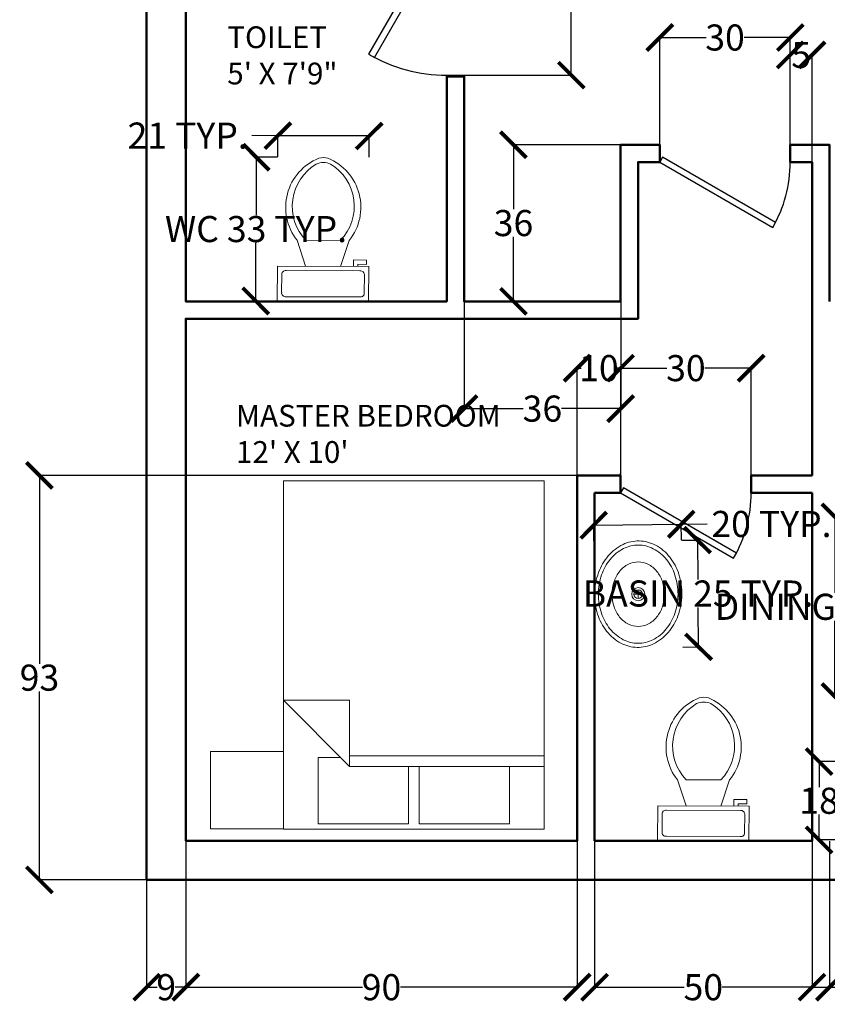
# Model space of a CAD drawing. Units: inches. Extents: x 9 to 573, y -373 to 44.
# Tile 1 of 5: x 9 to 195, y -373 to -146. Entities that reach past the tile are written whole.
import ezdxf

# ---------------------------------------------------------------- set-up
doc = ezdxf.new("R2010")
doc.units = ezdxf.units.IN
doc.header["$MEASUREMENT"] = 0
for name, color, linetype, lineweight in [('A-ANNO-DIMS', 2, 'Continuous', 18), ('A-AREA-IDEN', 7, 'Continuous', 25), ('A-DOOR', 4, 'Continuous', 25), ('A-FLOR-FIXT', 9, 'Continuous', 18), ('A-FURN', 8, 'Continuous', 18), ('A-WALL', 7, 'Continuous', 50)]:
    doc.layers.add(name, color=color, linetype=linetype, lineweight=lineweight)
doc.styles.get("Standard").update_dxf_attribs({"font": 'arial.ttf'})
doc.dimstyles.get("Standard").update_dxf_attribs({"dimtxt": 6, "dimasz": 6, "dimexe": 0.18, "dimexo": 0.0625, "dimgap": 0.09, "dimtad": 0, "dimtih": 1, "dimtoh": 1, "dimdec": 0, "dimzin": 0, "dimdsep": 46, "dimlunit": 4, "dimtxsty": 'Standard', "dimblk": 'ARCHTICK', "dimcen": 0.09, "dimadec": 0, "dimazin": 0, "dimtfac": 1, "dimtdec": 0, "dimtofl": 0, "dimtmove": 0, "dimatfit": 3, "dimldrblk": 'ARCHTICK', "dimfxl": 1, "dimtolj": 1, "dimtzin": 0, "dimarcsym": 0})

# ---------------------------------------------------------------- blocks, each defined once
blk = doc.blocks.new('*U6')
for p, q in [((0, 0), (0, 6)), ((40, 0), (40, 6))]:
    blk.add_line(p, q)
blk.add_lwpolyline([(0, 0), (34.64, -20), (35.52, -18.48), (0.87, 1.52)], close=True)
blk.add_arc((0, 0), 40, 330, 0)
blk = doc.blocks.new('Bed - Queen')
for p, q in [((0, -80.00003), (0, 0)), ((0, 0), (59.99999, 0)), ((59.99999, 0), (59.99999, -80.00003)), ((7.99999, -1.2), (28.79998, -1.2)), ((7.99999, -14.4), (7.99999, -1.2)), ((28.79998, -1.2), (28.79998, -14.4)), ((31.19999, -1.2), (51.99999, -1.2)), ((31.19999, -14.4), (31.19999, -1.2)), ((51.99999, -1.2), (51.99999, -16.4)), ((0, -14.4), (44.8, -14.4)), ((59.99999, -29.6), (44.8, -14.4)), ((44.8, -14.4), (44.8, -29.6)), ((44.8, -16.8), (0, -16.8)), ((51.99999, -16.4), (46.79936, -16.4)), ((44.8, -29.6), (59.99999, -29.6)), ((59.99999, -80.00003), (0, -80.00003))]:
    blk.add_line(p, q)
blk = doc.blocks.new('Sink - Oval top')
for p, q in [((-1, 0), (1, 0)), ((0, 1), (0, -1))]:
    blk.add_line(p, q)
for points in [[(-12.23, 0.39, 0.117634), (-11.46, -3.36, 0.104469), (-8.88, -6.8, 0.090016), (-5.08, -9.07, 0.08192), (-0.32, -10.02, 0.08192), (4.49, -9.38, 0.090016), (8.42, -7.36, 0.104469), (11.22, -4.09, 0.117634), (12.23, -0.39, 0.117634), (11.46, 3.36, 0.104469), (8.88, 6.8, 0.090016), (5.08, 9.07, 0.08192), (0.32, 10.02, 0.08192), (-4.49, 9.38, 0.090016), (-8.42, 7.36, 0.104469), (-11.22, 4.09, 0.117634)], [(-11.29, 0.16, 0.118622), (-10.52, -3.25, 0.104678), (-8.07, -6.36, 0.089562), (-4.54, -8.37, 0.081185), (-0.13, -9.15, 0.081185), (4.3, -8.49, 0.089562), (7.89, -6.58, 0.104678), (10.42, -3.55, 0.118622), (11.29, -0.16, 0.118622), (10.52, 3.25, 0.104678), (8.07, 6.36, 0.089562), (4.54, 8.37, 0.081185), (0.13, 9.15, 0.081185), (-4.3, 8.49, 0.089562), (-7.89, 6.58, 0.104678), (-10.42, 3.55, 0.118622)], [(-7.42, 0.08, 0.118283), (-6.91, -2.17, 0.104607), (-5.29, -4.21, 0.089718), (-2.97, -5.53, 0.081436), (-0.07, -6.04, 0.081436), (2.84, -5.59, 0.089718), (5.2, -4.33, 0.104607), (6.86, -2.32, 0.118283), (7.42, -0.08, 0.118283), (6.91, 2.17, 0.104607), (5.29, 4.21, 0.089718), (2.97, 5.53, 0.081436), (0.07, 6.04, 0.081436), (-2.84, 5.59, 0.089718), (-5.2, 4.33, 0.104607), (-6.86, 2.32, 0.118283)]]:
    blk.add_lwpolyline(points, format="xyb", close=True)
for radius in [1.5, 1]:
    blk.add_circle((0, 0), radius)
blk = doc.blocks.new('Toilet - top')
for p, q in [((9.5, -6), (9.5, -2)), ((-10, -8.5), (-8, -8.5)), ((-10, -9.5), (-10, -8.5)), ((-8, -8.5), (-8, -8)), ((-7, -8), (-7, -9.5)), ((-4, -8), (-6, -14)), ((4, -8), (6, -14)), ((-7, -9.5), (-10, -9.5)), ((4, -14), (-4, -14))]:
    blk.add_line(p, q)
blk.add_lwpolyline([(10.5, -8), (10.5, 0), (-10.5, 0), (-10.5, -8)], close=True)
for points in [[(-9.5, -2), (-9.5, -6)], [(8.5, -1), (-8.5, -1)], [(-8.5, -7), (8.5, -7)]]:
    blk.add_lwpolyline(points)
for centre, radius, start, end in [((-8.62, -1.88), 0.884, 81.8699, 188.1301), ((8.62, -1.88), 0.884, 351.8699, 98.1301), ((-8.62, -6.12), 0.884, 171.8699, 278.1301), ((8.62, -6.12), 0.884, 261.8699, 8.1301), ((3.52, -21.58), 12.17, 141.4691, 247.9714), ((4.2, -21.82), 11.33, 136.3677, 238.9468), ((-3.52, -21.58), 12.17, 292.0284, 38.5307), ((-4.2, -21.82), 11.33, 301.053, 43.6321), ((0, -27.88), 4, 245.7318, 294.2682), ((0, -29), 4, 254.8605, 285.1395)]:
    blk.add_arc(centre, radius, start, end)
blk = doc.blocks.new('*U25')
for p, q in [((0, 0), (0, 6)), ((40, 0), (40, 6))]:
    blk.add_line(p, q)
blk.add_lwpolyline([(0, 0), (34.64, -20), (35.52, -18.48), (0.87, 1.52)], close=True)
blk.add_arc((0, 0), 40, 330, 0)
blk = doc.blocks.new('BEDSIDE-TABLE')
blk.add_lwpolyline([(0, 17.82), (16.74, 17.82), (16.74, 0), (0, 0)], close=True)
blk = doc.blocks.new('_ArchTick')
at = {"color": 0, "linetype": 'ByBlock', "const_width": 0.15}
blk.add_lwpolyline([(-0.5, -0.5), (0.5, 0.5)], dxfattribs=at)
blk = doc.blocks.new('*D36')
at = {"layer": 'A-ANNO-DIMS', "color": 0, "lineweight": -2, "transparency": 16777216}
for p, q in [((68.61, -178.08), (63.54, -178.06)), ((63.72, -178.06), (63.67, -191.39)), ((63.6, -211.1), (63.65, -197.78)), ((68.49, -211.12), (63.42, -211.1))]:
    blk.add_line(p, q, dxfattribs=at)
at = {"layer": 'Defpoints', "color": 0, "transparency": 16777216}
for p in [(68.67, -178.08), (63.6, -211.1), (68.55, -211.12)]:
    blk.add_point(p, dxfattribs=at)
at = {"layer": 'A-ANNO-DIMS', "color": 0, "lineweight": -2, "transparency": 16777216, "xscale": 6, "yscale": 6, "zscale": 6}
for p, rotation in [((63.72, -178.06), 89.79498038757418), ((63.6, -211.1), 269.7949803875742)]:
    blk.add_blockref('_ArchTick', p, dxfattribs=dict(at, rotation=rotation))
at = {"layer": 'A-ANNO-DIMS', "color": 0, "transparency": 16777216, "insert": (63.66, -194.58), "char_height": 6, "attachment_point": 5}
blk.add_mtext('\\A1;WC 33 TYP.', dxfattribs=at)
blk = doc.blocks.new('*D37')
at = {"layer": 'A-ANNO-DIMS', "color": 0, "lineweight": -2, "transparency": 16777216}
for p, q in [((68.69, -173.12), (62.69, -173.1)), ((68.67, -178.01), (68.69, -172.94)), ((89.69, -173.19), (68.69, -173.12)), ((89.67, -178.09), (89.69, -173.01))]:
    blk.add_line(p, q, dxfattribs=at)
at = {"layer": 'Defpoints', "color": 0, "transparency": 16777216}
for p in [(68.69, -173.12), (68.67, -178.08), (89.67, -178.15)]:
    blk.add_point(p, dxfattribs=at)
at = {"layer": 'A-ANNO-DIMS', "color": 0, "lineweight": -2, "transparency": 16777216, "xscale": 6, "yscale": 6, "zscale": 6}
for p, rotation in [((68.69, -173.12), 179.7949803875742), ((89.69, -173.19), 359.7949803875743)]:
    blk.add_blockref('_ArchTick', p, dxfattribs=dict(at, rotation=rotation))
at = {"layer": 'A-ANNO-DIMS', "color": 0, "transparency": 16777216, "insert": (47.95, -173.1), "char_height": 6, "attachment_point": 5}
blk.add_mtext('\\A1;21 TYP.', dxfattribs=at)
blk = doc.blocks.new('*D38')
at = {"layer": 'A-ANNO-DIMS', "color": 0, "lineweight": -2, "transparency": 16777216}
for p, q in [((161.55, -266.12), (165.35, -266.08)), ((165.17, -266.08), (165.27, -275.16)), ((165.44, -290.63), (165.34, -281.55)), ((161.82, -290.67), (165.62, -290.63))]:
    blk.add_line(p, q, dxfattribs=at)
at = {"layer": 'Defpoints', "color": 0, "transparency": 16777216}
for p in [(161.49, -266.12), (161.76, -290.67), (165.44, -290.63)]:
    blk.add_point(p, dxfattribs=at)
at = {"layer": 'A-ANNO-DIMS', "color": 0, "lineweight": -2, "transparency": 16777216, "xscale": 6, "yscale": 6, "zscale": 6}
for p, rotation in [((165.17, -266.08), 90.63751015860011), ((165.44, -290.63), 270.6375101586001)]:
    blk.add_blockref('_ArchTick', p, dxfattribs=dict(at, rotation=rotation))
at = {"layer": 'A-ANNO-DIMS', "color": 0, "transparency": 16777216, "insert": (165.3, -278.36), "char_height": 6, "attachment_point": 5}
blk.add_mtext('\\A1;BASIN 25 TYP.', dxfattribs=at)
blk = doc.blocks.new('*D39')
at = {"layer": 'A-ANNO-DIMS', "color": 0, "lineweight": -2, "transparency": 16777216}
for p, q in [((141.31, -262.66), (161.44, -262.44)), ((141.35, -266.28), (141.31, -262.48)), ((161.48, -266.06), (161.44, -262.26)), ((161.44, -262.44), (167.44, -262.37))]:
    blk.add_line(p, q, dxfattribs=at)
at = {"layer": 'Defpoints', "color": 0, "transparency": 16777216}
for p in [(161.44, -262.44), (141.35, -266.35), (161.49, -266.12)]:
    blk.add_point(p, dxfattribs=at)
at = {"layer": 'A-ANNO-DIMS', "color": 0, "lineweight": -2, "transparency": 16777216, "xscale": 6, "yscale": 6, "zscale": 6}
for p, rotation in [((141.31, -262.66), 180.6375101586001), ((161.44, -262.44), 0.6375101586001275)]:
    blk.add_blockref('_ArchTick', p, dxfattribs=dict(at, rotation=rotation))
at = {"layer": 'A-ANNO-DIMS', "color": 0, "transparency": 16777216, "insert": (182.19, -262.37), "char_height": 6, "attachment_point": 5}
blk.add_mtext('\\A1;20 TYP.', dxfattribs=at)
blk = doc.blocks.new('*D46')
at = {"layer": 'A-ANNO-DIMS', "color": 0, "lineweight": -2, "transparency": 16777216}
for p, q in [((202.92, -260.76), (196.6, -260.76)), ((196.78, -260.76), (196.78, -278.22)), ((196.78, -302.06), (196.78, -284.61)), ((202.92, -302.06), (196.6, -302.06))]:
    blk.add_line(p, q, dxfattribs=at)
at = {"layer": 'Defpoints', "color": 0, "transparency": 16777216}
for p in [(202.98, -260.76), (196.78, -302.06), (202.98, -302.06)]:
    blk.add_point(p, dxfattribs=at)
at = {"layer": 'A-ANNO-DIMS', "color": 0, "lineweight": -2, "transparency": 16777216, "xscale": 6, "yscale": 6, "zscale": 6}
for p, rotation in [((196.78, -260.76), 90), ((196.78, -302.06), 270)]:
    blk.add_blockref('_ArchTick', p, dxfattribs=dict(at, rotation=rotation))
at = {"layer": 'A-ANNO-DIMS', "color": 0, "transparency": 16777216, "insert": (196.78, -281.41), "char_height": 6, "attachment_point": 5}
blk.add_mtext('\\A1;DINING SET 41', dxfattribs=at)
blk = doc.blocks.new('*D57')
at = {"layer": 'A-ANNO-DIMS', "color": 0, "lineweight": -2, "transparency": 16777216}
for p, q in [((198.49, -316.99), (192.97, -316.99)), ((193.15, -316.99), (193.15, -322.84)), ((193.15, -334.99), (193.15, -329.14)), ((198.49, -334.99), (192.97, -334.99))]:
    blk.add_line(p, q, dxfattribs=at)
at = {"layer": 'Defpoints', "color": 0, "transparency": 16777216}
for p in [(193.15, -316.99), (198.55, -316.99), (198.55, -334.99)]:
    blk.add_point(p, dxfattribs=at)
at = {"layer": 'A-ANNO-DIMS', "color": 0, "lineweight": -2, "transparency": 16777216, "xscale": 6, "yscale": 6, "zscale": 6}
for p, rotation in [((193.15, -316.99), 90), ((193.15, -334.99), 270)]:
    blk.add_blockref('_ArchTick', p, dxfattribs=dict(at, rotation=rotation))
at = {"layer": 'A-ANNO-DIMS', "color": 0, "transparency": 16777216, "insert": (193.15, -325.99), "char_height": 6, "attachment_point": 5}
blk.add_mtext('\\A1;18', dxfattribs=at)
blk = doc.blocks.new('*D60')
at = {"layer": 'A-ANNO-DIMS', "color": 0, "lineweight": -2, "transparency": 16777216}
for p, q in [((47.52, -335.26), (47.52, -369.03)), ((38.52, -344.26), (38.52, -369.03)), ((38.52, -368.85), (40.95, -368.85)), ((47.52, -368.85), (45.08, -368.85))]:
    blk.add_line(p, q, dxfattribs=at)
at = {"layer": 'Defpoints', "color": 0, "transparency": 16777216}
for p in [(47.52, -335.2), (38.52, -344.2), (38.52, -368.85)]:
    blk.add_point(p, dxfattribs=at)
at = {"layer": 'A-ANNO-DIMS', "color": 0, "lineweight": -2, "transparency": 16777216, "xscale": 6, "yscale": 6, "zscale": 6, "rotation": 180}
blk.add_blockref('_ArchTick', (38.52, -368.85), dxfattribs=at)
at = {"layer": 'A-ANNO-DIMS', "color": 0, "lineweight": -2, "transparency": 16777216, "xscale": 6, "yscale": 6, "zscale": 6}
blk.add_blockref('_ArchTick', (47.52, -368.85), dxfattribs=at)
at = {"layer": 'A-ANNO-DIMS', "color": 0, "transparency": 16777216, "insert": (43.02, -368.85), "char_height": 6, "attachment_point": 5}
blk.add_mtext('\\A1;9', dxfattribs=at)
blk = doc.blocks.new('*D61')
at = {"layer": 'A-ANNO-DIMS', "color": 0, "lineweight": -2, "transparency": 16777216}
for p, q in [((191.52, -335.26), (191.52, -369.03)), ((195.52, -335.26), (195.52, -369.03)), ((191.52, -368.85), (195.52, -368.85)), ((195.52, -368.85), (201.52, -368.85))]:
    blk.add_line(p, q, dxfattribs=at)
at = {"layer": 'Defpoints', "color": 0, "transparency": 16777216}
for p in [(191.52, -335.2), (195.52, -335.2), (195.52, -368.85)]:
    blk.add_point(p, dxfattribs=at)
at = {"layer": 'A-ANNO-DIMS', "color": 0, "lineweight": -2, "transparency": 16777216, "xscale": 6, "yscale": 6, "zscale": 6, "rotation": 180}
blk.add_blockref('_ArchTick', (191.52, -368.85), dxfattribs=at)
at = {"layer": 'A-ANNO-DIMS', "color": 0, "lineweight": -2, "transparency": 16777216, "xscale": 6, "yscale": 6, "zscale": 6}
blk.add_blockref('_ArchTick', (195.52, -368.85), dxfattribs=at)
at = {"layer": 'A-ANNO-DIMS', "color": 0, "transparency": 16777216, "insert": (203.68, -368.85), "char_height": 6, "attachment_point": 5}
blk.add_mtext('\\A1;4', dxfattribs=at)
blk = doc.blocks.new('*D62')
at = {"layer": 'A-ANNO-DIMS', "color": 0, "lineweight": -2, "transparency": 16777216}
for p, q in [((47.52, -335.26), (47.52, -369.03)), ((137.52, -335.26), (137.52, -369.03)), ((47.52, -368.85), (88.14, -368.85)), ((137.52, -368.85), (96.89, -368.85))]:
    blk.add_line(p, q, dxfattribs=at)
at = {"layer": 'Defpoints', "color": 0, "transparency": 16777216}
for p in [(47.52, -335.2), (137.52, -335.2), (137.52, -368.85)]:
    blk.add_point(p, dxfattribs=at)
at = {"layer": 'A-ANNO-DIMS', "color": 0, "lineweight": -2, "transparency": 16777216, "xscale": 6, "yscale": 6, "zscale": 6, "rotation": 180}
blk.add_blockref('_ArchTick', (47.52, -368.85), dxfattribs=at)
at = {"layer": 'A-ANNO-DIMS', "color": 0, "lineweight": -2, "transparency": 16777216, "xscale": 6, "yscale": 6, "zscale": 6}
blk.add_blockref('_ArchTick', (137.52, -368.85), dxfattribs=at)
at = {"layer": 'A-ANNO-DIMS', "color": 0, "transparency": 16777216, "insert": (92.52, -368.85), "char_height": 6, "attachment_point": 5}
blk.add_mtext('\\A1;90', dxfattribs=at)
blk = doc.blocks.new('*D63')
at = {"layer": 'A-ANNO-DIMS', "color": 0, "lineweight": -2, "transparency": 16777216}
for p, q in [((141.52, -335.26), (141.52, -369.03)), ((191.52, -335.26), (191.52, -369.03)), ((141.52, -368.85), (162.14, -368.85)), ((191.52, -368.85), (170.89, -368.85))]:
    blk.add_line(p, q, dxfattribs=at)
at = {"layer": 'Defpoints', "color": 0, "transparency": 16777216}
for p in [(141.52, -335.2), (191.52, -335.2), (191.52, -368.85)]:
    blk.add_point(p, dxfattribs=at)
at = {"layer": 'A-ANNO-DIMS', "color": 0, "lineweight": -2, "transparency": 16777216, "xscale": 6, "yscale": 6, "zscale": 6, "rotation": 180}
blk.add_blockref('_ArchTick', (141.52, -368.85), dxfattribs=at)
at = {"layer": 'A-ANNO-DIMS', "color": 0, "lineweight": -2, "transparency": 16777216, "xscale": 6, "yscale": 6, "zscale": 6}
blk.add_blockref('_ArchTick', (191.52, -368.85), dxfattribs=at)
at = {"layer": 'A-ANNO-DIMS', "color": 0, "transparency": 16777216, "insert": (166.52, -368.85), "char_height": 6, "attachment_point": 5}
blk.add_mtext('\\A1;50', dxfattribs=at)
blk = doc.blocks.new('*D64')
at = {"layer": 'A-ANNO-DIMS', "color": 0, "lineweight": -2, "transparency": 16777216}
for p, q in [((137.45, -251.2), (13.69, -251.2)), ((13.87, -251.2), (13.87, -294.54)), ((13.87, -344.2), (13.87, -300.85)), ((38.45, -344.2), (13.69, -344.2))]:
    blk.add_line(p, q, dxfattribs=at)
at = {"layer": 'Defpoints', "color": 0, "transparency": 16777216}
for p in [(13.87, -251.2), (137.52, -251.2), (38.52, -344.2)]:
    blk.add_point(p, dxfattribs=at)
at = {"layer": 'A-ANNO-DIMS', "color": 0, "lineweight": -2, "transparency": 16777216, "xscale": 6, "yscale": 6, "zscale": 6}
for p, rotation in [((13.87, -251.2), 90), ((13.87, -344.2), 270)]:
    blk.add_blockref('_ArchTick', p, dxfattribs=dict(at, rotation=rotation))
at = {"layer": 'A-ANNO-DIMS', "color": 0, "transparency": 16777216, "insert": (13.87, -297.7), "char_height": 6, "attachment_point": 5}
blk.add_mtext('\\A1;93', dxfattribs=at)
blk = doc.blocks.new('*D76')
at = {"layer": 'A-ANNO-DIMS', "color": 0, "lineweight": -2, "transparency": 16777216}
for p, q in [((147.45, -175.2), (122.69, -175.2)), ((122.87, -175.2), (122.87, -190.04)), ((122.87, -211.2), (122.87, -196.35)), ((147.45, -211.2), (122.69, -211.2))]:
    blk.add_line(p, q, dxfattribs=at)
at = {"layer": 'Defpoints', "color": 0, "transparency": 16777216}
for p in [(122.87, -175.2), (147.52, -175.2), (147.52, -211.2)]:
    blk.add_point(p, dxfattribs=at)
at = {"layer": 'A-ANNO-DIMS', "color": 0, "lineweight": -2, "transparency": 16777216, "xscale": 6, "yscale": 6, "zscale": 6}
for p, rotation in [((122.87, -175.2), 90), ((122.87, -211.2), 270)]:
    blk.add_blockref('_ArchTick', p, dxfattribs=dict(at, rotation=rotation))
at = {"layer": 'A-ANNO-DIMS', "color": 0, "transparency": 16777216, "insert": (122.87, -193.2), "char_height": 6, "attachment_point": 5}
blk.add_mtext('\\A1;36', dxfattribs=at)
blk = doc.blocks.new('*D77')
at = {"layer": 'A-ANNO-DIMS', "color": 0, "lineweight": -2, "transparency": 16777216}
for p, q in [((111.52, -211.26), (111.52, -236.03)), ((147.52, -211.26), (147.52, -236.03)), ((111.52, -235.85), (125.13, -235.85)), ((147.52, -235.85), (133.9, -235.85))]:
    blk.add_line(p, q, dxfattribs=at)
at = {"layer": 'Defpoints', "color": 0, "transparency": 16777216}
for p in [(111.52, -211.2), (147.52, -211.2), (111.52, -235.85)]:
    blk.add_point(p, dxfattribs=at)
at = {"layer": 'A-ANNO-DIMS', "color": 0, "lineweight": -2, "transparency": 16777216, "xscale": 6, "yscale": 6, "zscale": 6, "rotation": 180}
blk.add_blockref('_ArchTick', (111.52, -235.85), dxfattribs=at)
at = {"layer": 'A-ANNO-DIMS', "color": 0, "lineweight": -2, "transparency": 16777216, "xscale": 6, "yscale": 6, "zscale": 6}
blk.add_blockref('_ArchTick', (147.52, -235.85), dxfattribs=at)
at = {"layer": 'A-ANNO-DIMS', "color": 0, "transparency": 16777216, "insert": (129.52, -235.85), "char_height": 6, "attachment_point": 5}
blk.add_mtext('\\A1;36', dxfattribs=at)
blk = doc.blocks.new('*D78')
at = {"layer": 'A-ANNO-DIMS', "color": 0, "lineweight": -2, "transparency": 16777216}
for p, q in [((156.52, -175.13), (156.52, -150.37)), ((156.52, -150.55), (167.14, -150.55)), ((186.52, -150.55), (175.89, -150.55)), ((186.52, -175.13), (186.52, -150.37))]:
    blk.add_line(p, q, dxfattribs=at)
at = {"layer": 'Defpoints', "color": 0, "transparency": 16777216}
for p in [(186.52, -150.55), (156.52, -175.2), (186.52, -175.2)]:
    blk.add_point(p, dxfattribs=at)
at = {"layer": 'A-ANNO-DIMS', "color": 0, "lineweight": -2, "transparency": 16777216, "xscale": 6, "yscale": 6, "zscale": 6, "rotation": 180}
blk.add_blockref('_ArchTick', (156.52, -150.55), dxfattribs=at)
at = {"layer": 'A-ANNO-DIMS', "color": 0, "lineweight": -2, "transparency": 16777216, "xscale": 6, "yscale": 6, "zscale": 6}
blk.add_blockref('_ArchTick', (186.52, -150.55), dxfattribs=at)
at = {"layer": 'A-ANNO-DIMS', "color": 0, "transparency": 16777216, "insert": (171.52, -150.55), "char_height": 6, "attachment_point": 5}
blk.add_mtext('\\A1;30', dxfattribs=at)
blk = doc.blocks.new('*D79')
at = {"layer": 'A-ANNO-DIMS', "color": 0, "lineweight": -2, "transparency": 16777216}
for p, q in [((186.52, -179.13), (186.52, -154.37)), ((186.52, -154.55), (186.94, -154.55)), ((191.52, -154.55), (191.1, -154.55)), ((191.52, -179.13), (191.52, -154.37))]:
    blk.add_line(p, q, dxfattribs=at)
at = {"layer": 'Defpoints', "color": 0, "transparency": 16777216}
for p in [(191.52, -154.55), (186.52, -179.2), (191.52, -179.2)]:
    blk.add_point(p, dxfattribs=at)
at = {"layer": 'A-ANNO-DIMS', "color": 0, "lineweight": -2, "transparency": 16777216, "xscale": 6, "yscale": 6, "zscale": 6, "rotation": 180}
blk.add_blockref('_ArchTick', (186.52, -154.55), dxfattribs=at)
at = {"layer": 'A-ANNO-DIMS', "color": 0, "lineweight": -2, "transparency": 16777216, "xscale": 6, "yscale": 6, "zscale": 6}
blk.add_blockref('_ArchTick', (191.52, -154.55), dxfattribs=at)
at = {"layer": 'A-ANNO-DIMS', "color": 0, "transparency": 16777216, "insert": (189.02, -154.55), "char_height": 6, "attachment_point": 5}
blk.add_mtext('\\A1;5', dxfattribs=at)
blk = doc.blocks.new('*D80')
at = {"layer": 'A-ANNO-DIMS', "color": 0, "lineweight": -2, "transparency": 16777216}
for p, q in [((111.58, -123.2), (136.35, -123.2)), ((136.17, -123.2), (136.17, -138.04)), ((136.17, -159.2), (136.17, -144.35)), ((111.58, -159.2), (136.35, -159.2))]:
    blk.add_line(p, q, dxfattribs=at)
at = {"layer": 'Defpoints', "color": 0, "transparency": 16777216}
for p in [(111.52, -123.2), (111.52, -159.2), (136.17, -159.2)]:
    blk.add_point(p, dxfattribs=at)
at = {"layer": 'A-ANNO-DIMS', "color": 0, "lineweight": -2, "transparency": 16777216, "xscale": 6, "yscale": 6, "zscale": 6}
for p, rotation in [((136.17, -123.2), 90), ((136.17, -159.2), 270)]:
    blk.add_blockref('_ArchTick', p, dxfattribs=dict(at, rotation=rotation))
at = {"layer": 'A-ANNO-DIMS', "color": 0, "transparency": 16777216, "insert": (136.17, -141.2), "char_height": 6, "attachment_point": 5}
blk.add_mtext('\\A1;36', dxfattribs=at)
blk = doc.blocks.new('*D86')
at = {"layer": 'A-ANNO-DIMS', "color": 0, "lineweight": -2, "transparency": 16777216}
for p, q in [((147.52, -251.13), (147.52, -226.37)), ((147.52, -226.55), (158.14, -226.55)), ((177.52, -226.55), (166.89, -226.55)), ((177.52, -251.13), (177.52, -226.37))]:
    blk.add_line(p, q, dxfattribs=at)
at = {"layer": 'Defpoints', "color": 0, "transparency": 16777216}
for p in [(177.52, -226.55), (147.52, -251.2), (177.52, -251.2)]:
    blk.add_point(p, dxfattribs=at)
at = {"layer": 'A-ANNO-DIMS', "color": 0, "lineweight": -2, "transparency": 16777216, "xscale": 6, "yscale": 6, "zscale": 6, "rotation": 180}
blk.add_blockref('_ArchTick', (147.52, -226.55), dxfattribs=at)
at = {"layer": 'A-ANNO-DIMS', "color": 0, "lineweight": -2, "transparency": 16777216, "xscale": 6, "yscale": 6, "zscale": 6}
blk.add_blockref('_ArchTick', (177.52, -226.55), dxfattribs=at)
at = {"layer": 'A-ANNO-DIMS', "color": 0, "transparency": 16777216, "insert": (162.52, -226.55), "char_height": 6, "attachment_point": 5}
blk.add_mtext('\\A1;30', dxfattribs=at)
blk = doc.blocks.new('*D87')
at = {"layer": 'A-ANNO-DIMS', "color": 0, "lineweight": -2, "transparency": 16777216}
for p, q in [((137.52, -251.13), (137.52, -226.37)), ((137.52, -226.55), (138.42, -226.55)), ((147.52, -226.55), (146.61, -226.55)), ((147.52, -251.13), (147.52, -226.37))]:
    blk.add_line(p, q, dxfattribs=at)
at = {"layer": 'Defpoints', "color": 0, "transparency": 16777216}
for p in [(147.52, -226.55), (137.52, -251.2), (147.52, -251.2)]:
    blk.add_point(p, dxfattribs=at)
at = {"layer": 'A-ANNO-DIMS', "color": 0, "lineweight": -2, "transparency": 16777216, "xscale": 6, "yscale": 6, "zscale": 6, "rotation": 180}
blk.add_blockref('_ArchTick', (137.52, -226.55), dxfattribs=at)
at = {"layer": 'A-ANNO-DIMS', "color": 0, "lineweight": -2, "transparency": 16777216, "xscale": 6, "yscale": 6, "zscale": 6}
blk.add_blockref('_ArchTick', (147.52, -226.55), dxfattribs=at)
at = {"layer": 'A-ANNO-DIMS', "color": 0, "transparency": 16777216, "insert": (142.52, -226.55), "char_height": 6, "attachment_point": 5}
blk.add_mtext('\\A1;10', dxfattribs=at)

msp = doc.modelspace()

# ---------------------------------------------------------------- linework, layer by layer
at = {"layer": 'A-WALL'}
for p, q in [((111.5169, -159.4915), (107.5169, -159.4915)), ((186.5169, -175.1966), (186.5169, -179.1966)), ((147.5169, -251.1966), (137.5169, -251.1966)), ((147.5169, -255.1966), (147.5169, -251.1966)), ((191.5169, -251.1966), (177.5169, -251.1966)), ((177.5169, -255.1966), (177.5169, -251.1966)), ((147.5169, -255.1966), (141.5169, -255.1966)), ((191.5169, -255.1966), (177.5169, -255.1966))]:
    msp.add_line(p, q, dxfattribs=at)
for points in [[(329.5169, -215.1966), (329.5169, -335.1966), (509.5169, -335.1966), (518.5169, -335.1966), (518.5169, -344.1966), (38.5169, -344.1966), (38.5169, 15.8034), (518.5169, 15.8034), (518.5169, -117.1966), (450.7536, -117.1966), (450.7536, -140.1966), (446.7536, -140.1966), (446.7536, -117.1966), (431.5169, -117.1966), (431.5169, -113.1966), (509.5169, -113.1966), (509.5169, 6.8034), (389.5169, 6.8034), (389.5169, -113.1966), (395.5169, -113.1966), (395.5169, -117.1966), (385.5169, -117.1966), (385.5169, 6.8034), (325.5169, 6.8034)], [(47.5169, -117.1966), (47.5169, -211.1966), (107.5169, -211.1966), (107.5169, -159.1966)], [(111.5169, -159.1966), (111.5169, -211.1966), (147.5169, -211.1966), (147.5169, -175.1966), (151.5169, -175.1966), (156.5169, -175.1966), (156.5169, -179.1966), (151.5169, -179.1966), (151.5169, -215.1966), (47.5169, -215.1966), (47.5169, -335.1966), (137.5169, -335.1966), (137.5169, -251.1966)], [(195.5169, -211.1966), (195.5169, -175.1966), (186.5169, -175.1966)], [(186.5169, -179.1966), (191.5169, -179.1966), (191.5169, -251.1966)], [(191.5169, -255.1966), (191.5169, -335.1966), (141.5169, -335.1966), (141.5169, -255.1966)]]:
    msp.add_lwpolyline(points, dxfattribs=at)

# ---------------------------------------------------------------- block references
at = {"layer": 'A-DOOR', "xscale": 0.9, "yscale": 0.9, "zscale": 0.9, "rotation": 270}
msp.add_blockref('*U25', (107.5169, -123.1966), dxfattribs=at)
at = {"layer": 'A-DOOR', "xscale": 0.75, "yscale": 0.75, "zscale": 0.75}
for p in [(156.5169, -179.1966), (147.5169, -255.1966)]:
    msp.add_blockref('*U6', p, dxfattribs=at)
at = {"layer": 'A-FLOR-FIXT'}
for name, p, rotation in [('Toilet - top', (79.0545, -211.159), 179.7949803875742), ('Sink - Oval top', (151.5546, -278.5082), 270.6375101586001), ('Toilet - top', (166.5169, -335.1966), 179.7949803875742)]:
    msp.add_blockref(name, p, dxfattribs=dict(at, rotation=rotation))
at = {"layer": 'A-FURN', "rotation": 180}
for name, p in [('Bed - Queen', (129.9624, -332.4892)), ('BEDSIDE-TABLE', (69.9629, -314.6647))]:
    msp.add_blockref(name, p, dxfattribs=at)

# ---------------------------------------------------------------- texts
at = {"layer": 'A-AREA-IDEN', "char_height": 5, "attachment_point": 1}
for s, width, insert in [('TOILET \\P5\' X 7\'9"', 36.887692, (57.0545, -147.9915)), ("MASTER BEDROOM\\P12' X 10'", 117.44018, (59.0545, -234.9915))]:
    msp.add_mtext_dynamic_manual_height_columns(s, width=width, gutter_width=1, heights=[0], dxfattribs=dict(at, insert=insert))

# ---------------------------------------------------------------- dimensions: what is measured, and where the dimension line sits
at = {"layer": 'A-ANNO-DIMS'}
for base, p1, p2, angle, picture, middle in [((136.1669, -159.1966), (111.5169, -123.1966), (111.5169, -159.1966), 270, '*D80', (136.1669, -141.1966)), ((122.8669, -175.1966), (147.5169, -211.1966), (147.5169, -175.1966), 90, '*D76', (122.8669, -193.1966)), ((111.5169, -235.8466), (147.5169, -211.1966), (111.5169, -211.1966), 180, '*D77', (129.5169, -235.8466)), ((13.8669, -251.1966), (38.5169, -344.1966), (137.5169, -251.1966), 90, '*D64', (13.8669, -297.6966)), ((193.1545, -316.9915), (198.5545, -334.9915), (198.5545, -316.9915), 90, '*D57', (193.1545, -325.9915))]:
    dim = msp.add_linear_dim(base=base, p1=p1, p2=p2, angle=angle, dimstyle='Standard', override={"dimdec": 0, "dimlfac": 1, "dimrnd": 0, "dimzin": 0, "dimdsep": 46, "dimlunit": 2}, dxfattribs=at)
    dim.commit()
    dim.dimension.update_dxf_attribs({"geometry": picture, "text_midpoint": middle})
for base, p1, p2, picture, middle in [((186.5169, -150.5466), (156.5169, -175.1966), (186.5169, -175.1966), '*D78', (171.5169, -150.5466)), ((191.5169, -154.5466), (186.5169, -179.1966), (191.5169, -179.1966), '*D79', (189.0169, -154.5466)), ((147.5169, -226.5466), (137.5169, -251.1966), (147.5169, -251.1966), '*D87', (142.5169, -226.5466)), ((177.5169, -226.5466), (147.5169, -251.1966), (177.5169, -251.1966), '*D86', (162.5169, -226.5466)), ((38.5169, -368.8466), (47.5169, -335.1966), (38.5169, -344.1966), '*D60', (43.0169, -368.8466)), ((137.5169, -368.8466), (47.5169, -335.1966), (137.5169, -335.1966), '*D62', (92.5169, -368.8466)), ((191.5169, -368.8466), (141.5169, -335.1966), (191.5169, -335.1966), '*D63', (166.5169, -368.8466)), ((195.5169, -368.8466), (191.5169, -335.1966), (195.5169, -335.1966), '*D61', (203.6819, -368.8466))]:
    dim = msp.add_linear_dim(base=base, p1=p1, p2=p2, dimstyle='Standard', override={"dimdec": 0, "dimlfac": 1, "dimrnd": 0, "dimzin": 0, "dimdsep": 46, "dimlunit": 2}, dxfattribs=at)
    dim.commit()
    dim.dimension.update_dxf_attribs({"geometry": picture, "text_midpoint": middle})
for base, p1, p2, angle, text, picture, middle in [((68.6906, -173.1185), (89.6727, -178.1506), (68.6728, -178.0754), 179.79498, '<> TYP.', '*D37', (47.9465, -173.0971)), ((63.5977, -211.1037), (68.6728, -178.0754), (68.5546, -211.1215), 269.79498, 'WC <> TYP.', '*D36', (63.6568, -194.5807)), ((161.4447, -262.4391), (141.3503, -266.3455), (161.4856, -266.1215), 0.63751, '<> TYP.', '*D39', (182.1885, -262.3723)), ((196.7832, -302.0645), (202.9786, -260.7621), (202.9786, -302.0645), 270, 'DINING SET <>', '*D46', (196.7832, -281.4133)), ((165.4412, -290.6299), (161.4856, -266.1215), (161.7588, -290.6708), 270.63751, 'BASIN <> TYP.', '*D38', (165.3046, -278.3552))]:
    dim = msp.add_linear_dim(base=base, p1=p1, p2=p2, angle=angle, text=text, dimstyle='Standard', override={"dimdec": 0, "dimlfac": 1, "dimrnd": 0, "dimzin": 0, "dimdsep": 46, "dimlunit": 2}, dxfattribs=at)
    dim.commit()
    dim.dimension.update_dxf_attribs({"geometry": picture, "text_midpoint": middle})

doc.saveas('drawing.dxf')
